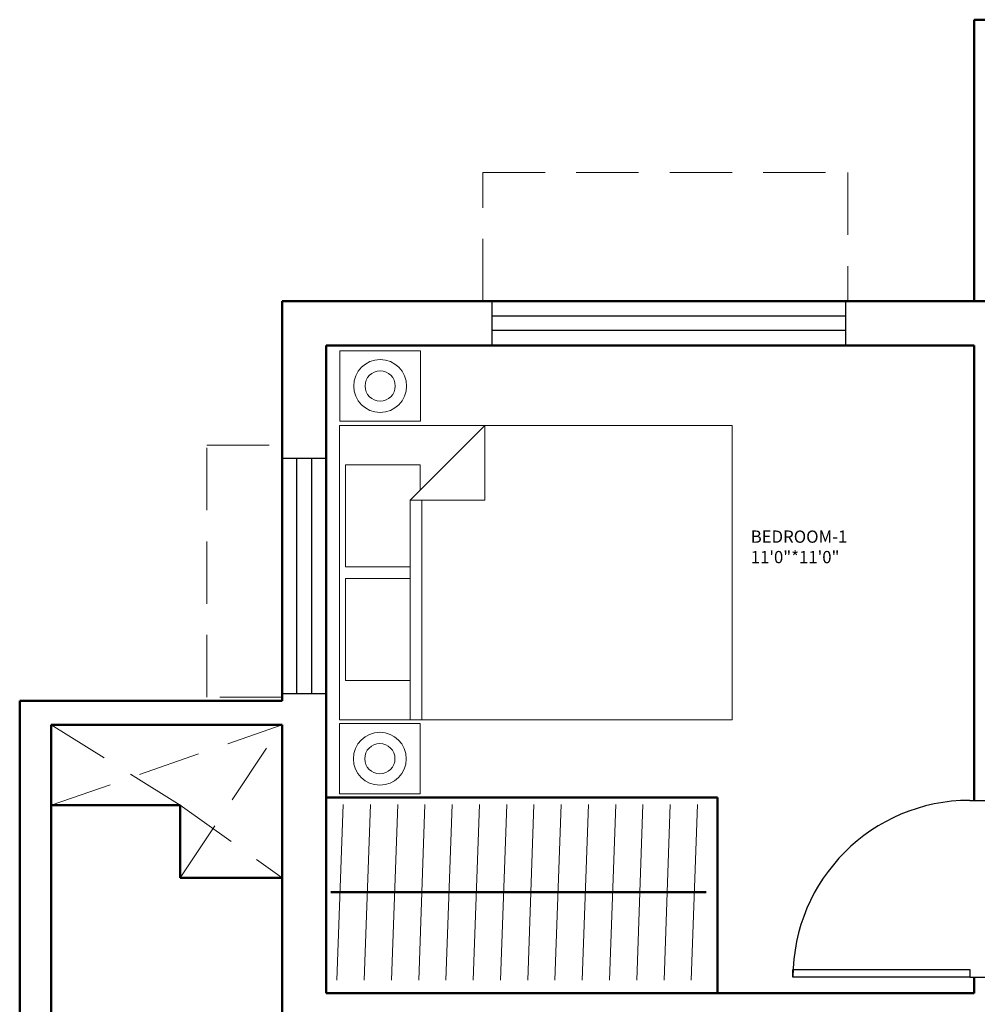
# Model space of a CAD drawing. Units: inches. Extents: x 291 to 2631, y 456 to 2623.
# Tile 15 of 22: x 1501 to 1696, y 2022 to 2223. Entities that reach past the tile are written whole.
import ezdxf

# ---------------------------------------------------------------- set-up
doc = ezdxf.new("R2010")
doc.units = ezdxf.units.IN
doc.linetypes.add('DASHED', pattern=[19.05, 12.7, -6.35])
for name, color, linetype, lineweight in [('A-AREA-IDEN', 7, 'Continuous', 25), ('A-DOOR', 3, 'Continuous', 25), ('A-FLOR-OVHD', 1, 'DASHED', 18), ('A-FURN', 8, 'Continuous', 18), ('A-GLAZ', 4, 'Continuous', 25), ('A-WALL', 7, 'Continuous', 50)]:
    doc.layers.add(name, color=color, linetype=linetype, lineweight=lineweight)
doc.styles.get("Standard").update_dxf_attribs({"font": 'arial.ttf'})

# ---------------------------------------------------------------- blocks, each defined once
blk = doc.blocks.new('*U2')
for p, q in [((0, 0), (0, -6)), ((40, 0), (40, -6))]:
    blk.add_line(p, q)
blk.add_lwpolyline([(0, 0), (0, 40), (1.75, 40), (1.75, 0)], close=True)
blk.add_arc((0, 0), 40, 0, 90)
blk = doc.blocks.new('Bed - Queen')
for p, q in [((0, -80.00003), (0, 0)), ((0, 0), (59.99999, 0)), ((59.99999, 0), (59.99999, -80.00003)), ((7.99999, -1.2), (28.79998, -1.2)), ((7.99999, -14.4), (7.99999, -1.2)), ((28.79998, -1.2), (28.79998, -14.4)), ((31.19999, -1.2), (51.99999, -1.2)), ((31.19999, -14.4), (31.19999, -1.2)), ((51.99999, -1.2), (51.99999, -16.4)), ((0, -14.4), (44.8, -14.4)), ((59.99999, -29.6), (44.8, -14.4)), ((44.8, -14.4), (44.8, -29.6)), ((44.8, -16.8), (0, -16.8)), ((51.99999, -16.4), (46.79936, -16.4)), ((44.8, -29.6), (59.99999, -29.6)), ((59.99999, -80.00003), (0, -80.00003))]:
    blk.add_line(p, q)
blk = doc.blocks.new('WIN-1800')
for p, q in [((0, 9), (72, 9)), ((0, 0), (0, 9)), ((72, 9), (72, 0)), ((0, 6), (72, 6)), ((72, 3), (0, 3)), ((72, 0), (0, 0))]:
    blk.add_line(p, q)
blk = doc.blocks.new('WIN-1200')
for p, q in [((0, 0), (0, 48)), ((0, 48), (9, 48)), ((3, 0), (3, 48)), ((6, 48), (6, 0)), ((9, 48), (9, 0)), ((9, 0), (0, 0))]:
    blk.add_line(p, q)

msp = doc.modelspace()

# ---------------------------------------------------------------- linework, layer by layer
at = {"layer": 'A-FLOR-OVHD'}
for p, q in [((1595.39, 2165.24), (1595.39, 2191.45)), ((1595.39, 2191.45), (1669.74, 2191.45)), ((1669.74, 2191.45), (1669.74, 2165.24)), ((1539.16, 2084.53), (1539.16, 2135.89)), ((1539.16, 2135.89), (1554.49, 2135.89)), ((1554.49, 2084.53), (1539.16, 2084.53)), ((1507.45, 2062.56), (1554.49, 2078.92)), ((1507.45, 2078.92), (1533.75, 2062.56)), ((1533.75, 2047.76), (1554.49, 2078.92)), ((1533.75, 2062.56), (1554.49, 2047.76))]:
    msp.add_line(p, q, dxfattribs=at)
at = {"layer": 'A-FURN'}
for p, q in [((1565.67, 2026.92), (1566.94, 2062.7)), ((1571.22, 2026.92), (1572.49, 2062.7)), ((1576.78, 2026.92), (1578.04, 2062.7)), ((1582.33, 2026.92), (1583.6, 2062.7)), ((1587.88, 2026.92), (1589.15, 2062.7)), ((1593.44, 2026.92), (1594.7, 2062.7)), ((1598.99, 2026.92), (1600.25, 2062.7)), ((1604.54, 2026.92), (1605.81, 2062.7)), ((1610.09, 2026.92), (1611.36, 2062.7)), ((1615.65, 2026.92), (1616.91, 2062.7)), ((1621.2, 2026.92), (1622.47, 2062.7)), ((1626.75, 2026.92), (1628.02, 2062.7)), ((1632.31, 2026.92), (1633.57, 2062.7)), ((1637.86, 2026.92), (1639.12, 2062.7))]:
    msp.add_line(p, q, dxfattribs=at)
for points in [[(1566.23, 2155.11), (1582.71, 2155.11), (1582.71, 2140.81), (1566.23, 2140.81)], [(1566.17, 2079.17), (1582.65, 2079.17), (1582.65, 2064.88), (1566.17, 2064.88)]]:
    msp.add_lwpolyline(points, close=True, dxfattribs=at)
for centre, radius in [((1574.47, 2147.96), 5.39), ((1574.47, 2147.96), 3.08), ((1574.41, 2072.02), 5.39), ((1574.41, 2072.02), 3.08)]:
    msp.add_circle(centre, radius, dxfattribs=at)
at = {"layer": 'A-WALL'}
for p, q in [((1695.49, 2165.24), (1695.49, 2222.59)), ((1695.49, 2222.59), (1699.99, 2222.59)), ((1554.49, 2165.24), (1554.49, 2083.8)), ((1699.99, 2165.24), (1554.49, 2165.24)), ((1563.49, 2156.24), (1563.49, 2024.24)), ((1695.49, 2156.24), (1563.49, 2156.24)), ((1695.49, 2156.24), (1695.49, 2063.53)), ((1554.49, 2083.8), (1501.02, 2083.8)), ((1501.02, 2083.8), (1501.02, 1959.74)), ((1554.49, 2078.92), (1507.45, 2078.92)), ((1507.45, 2078.92), (1507.45, 1959.74)), ((1554.49, 2078.92), (1554.49, 1959.74)), ((1507.45, 2062.56), (1533.75, 2062.56)), ((1533.75, 2062.56), (1533.75, 2047.76)), ((1563.49, 2064.11), (1643.2, 2064.11)), ((1643.2, 2064.11), (1643.2, 2024.24)), ((1533.75, 2047.76), (1554.49, 2047.76)), ((1564.42, 2044.81), (1640.87, 2044.81)), ((1695.49, 2027.53), (1695.49, 2024.24)), ((1695.49, 2024.24), (1563.49, 2024.24))]:
    msp.add_line(p, q, dxfattribs=at)

# ---------------------------------------------------------------- block references
at = {"layer": 'A-DOOR', "xscale": 0.9, "yscale": 0.9, "zscale": 0.9, "rotation": 90}
msp.add_blockref('*U2', (1694.59, 2027.53), dxfattribs=at)
at = {"layer": 'A-FURN', "rotation": 90}
msp.add_blockref('Bed - Queen', (1566.19, 2079.93), dxfattribs=at)
at = {"layer": 'A-GLAZ'}
for name, p in [('WIN-1800', (1597.3, 2156.24)), ('WIN-1200', (1554.49, 2085.26))]:
    msp.add_blockref(name, p, dxfattribs=at)

# ---------------------------------------------------------------- texts
at = {"layer": 'A-AREA-IDEN', "insert": (1649.98, 2118.52), "char_height": 2.5, "attachment_point": 1}
msp.add_mtext_dynamic_manual_height_columns('BEDROOM-1\\P11\'0"*11\'0"', width=40.393, gutter_width=12.5, heights=[0], dxfattribs=at)

doc.saveas('drawing.dxf')
